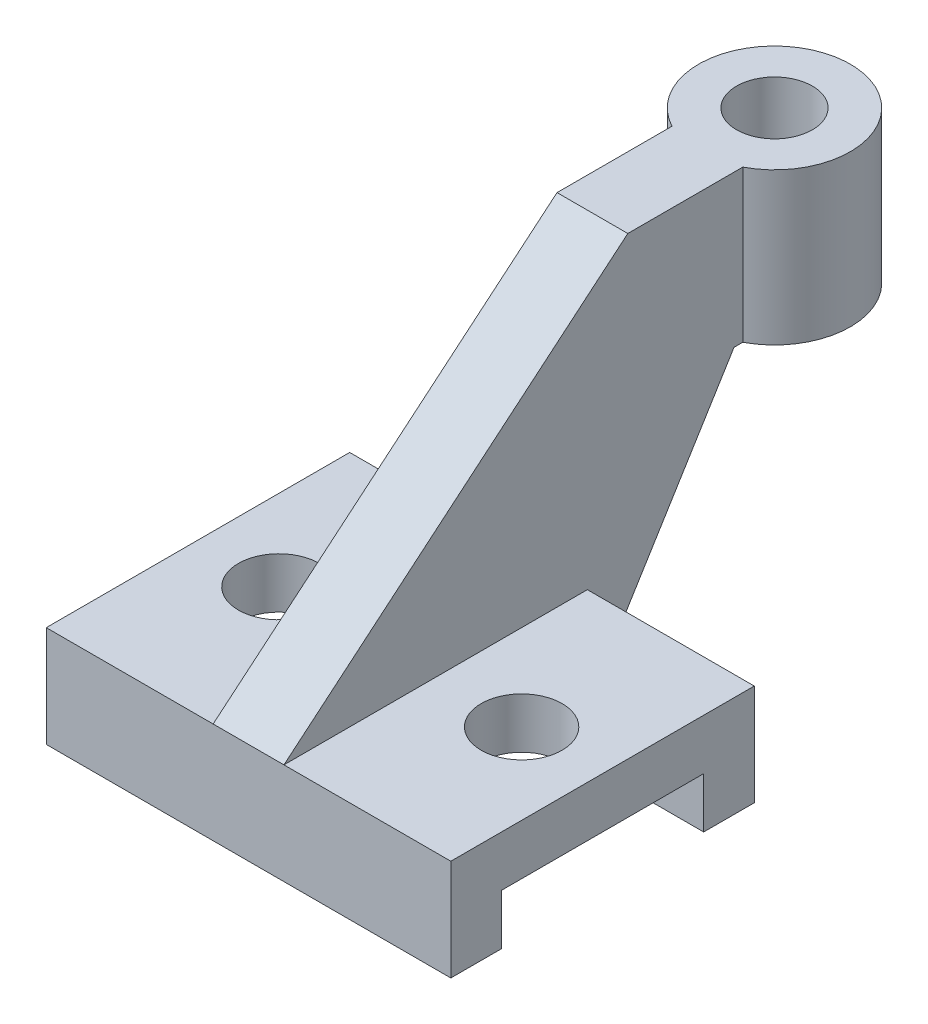
ISO-10303-21;
HEADER;
FILE_DESCRIPTION(('STEP AP214'),'2;1');
FILE_NAME('part.step','',(''),(''),'','','');
FILE_SCHEMA(('AUTOMOTIVE_DESIGN { 1 0 10303 214 1 1 1 1 }'));
ENDSEC;
DATA;
#1=APPLICATION_CONTEXT('core data for automotive mechanical design processes');
#2=APPLICATION_PROTOCOL_DEFINITION('international standard','automotive_design',2000,#1);
#3=PRODUCT_CONTEXT('',#1,'mechanical');
#4=PRODUCT('Part','Part','',(#3));
#5=PRODUCT_RELATED_PRODUCT_CATEGORY('part','',(#4));
#6=PRODUCT_DEFINITION_FORMATION('','',#4);
#7=PRODUCT_DEFINITION_CONTEXT('part definition',#1,'design');
#8=PRODUCT_DEFINITION('design','',#6,#7);
#9=PRODUCT_DEFINITION_SHAPE('','',#8);
#10=(LENGTH_UNIT() NAMED_UNIT(*) SI_UNIT(.MILLI.,.METRE.));
#11=(NAMED_UNIT(*) PLANE_ANGLE_UNIT() SI_UNIT($,.RADIAN.));
#12=(NAMED_UNIT(*) SI_UNIT($,.STERADIAN.) SOLID_ANGLE_UNIT());
#13=UNCERTAINTY_MEASURE_WITH_UNIT(LENGTH_MEASURE(1.E-05),#10,'distance_accuracy_value','');
#14=(GEOMETRIC_REPRESENTATION_CONTEXT(3) GLOBAL_UNCERTAINTY_ASSIGNED_CONTEXT((#13)) GLOBAL_UNIT_ASSIGNED_CONTEXT((#10,
#11,#12)) REPRESENTATION_CONTEXT('',''));
#15=CARTESIAN_POINT('',(0.,0.,0.));
#16=DIRECTION('',(0.,0.,1.));
#17=DIRECTION('',(1.,0.,0.));
#18=AXIS2_PLACEMENT_3D('',#15,#16,#17);
#19=CARTESIAN_POINT('',(-40.,-10.,30.));
#20=DIRECTION('',(0.,1.,0.));
#21=DIRECTION('',(0.,0.,1.));
#22=AXIS2_PLACEMENT_3D('',#19,#20,#21);
#23=PLANE('',#22);
#24=DIRECTION('',(1.,0.,0.));
#25=VECTOR('',#24,1.);
#26=CARTESIAN_POINT('',(-40.,-10.,-20.));
#27=LINE('',#26,#25);
#28=CARTESIAN_POINT('',(-40.,-10.,-20.));
#29=VERTEX_POINT('',#28);
#30=CARTESIAN_POINT('',(40.,-10.,-20.));
#31=VERTEX_POINT('',#30);
#32=EDGE_CURVE('E154',#29,#31,#27,.T.);
#33=ORIENTED_EDGE('',*,*,#32,.F.);
#34=DIRECTION('',(0.,0.,-1.));
#35=VECTOR('',#34,1.);
#36=CARTESIAN_POINT('',(-40.,-10.,30.));
#37=LINE('',#36,#35);
#38=CARTESIAN_POINT('',(-40.,-10.,-30.));
#39=VERTEX_POINT('',#38);
#40=EDGE_CURVE('E172',#29,#39,#37,.T.);
#41=ORIENTED_EDGE('',*,*,#40,.T.);
#42=DIRECTION('',(1.,0.,0.));
#43=VECTOR('',#42,1.);
#44=CARTESIAN_POINT('',(-40.,-10.,-30.));
#45=LINE('',#44,#43);
#46=CARTESIAN_POINT('',(-7.,-10.,-30.));
#47=VERTEX_POINT('',#46);
#48=EDGE_CURVE('E269',#39,#47,#45,.T.);
#49=ORIENTED_EDGE('',*,*,#48,.T.);
#50=DIRECTION('',(-1.,0.,0.));
#51=VECTOR('',#50,1.);
#52=CARTESIAN_POINT('',(7.,-10.,-30.));
#53=LINE('',#52,#51);
#54=CARTESIAN_POINT('',(7.,-10.,-30.));
#55=VERTEX_POINT('',#54);
#56=EDGE_CURVE('E265',#55,#47,#53,.T.);
#57=ORIENTED_EDGE('',*,*,#56,.F.);
#58=CARTESIAN_POINT('',(40.,-10.,-30.));
#59=VERTEX_POINT('',#58);
#60=EDGE_CURVE('E286',#55,#59,#45,.T.);
#61=ORIENTED_EDGE('',*,*,#60,.T.);
#62=DIRECTION('',(0.,0.,-1.));
#63=VECTOR('',#62,1.);
#64=CARTESIAN_POINT('',(40.,-10.,30.));
#65=LINE('',#64,#63);
#66=EDGE_CURVE('E280',#31,#59,#65,.T.);
#67=ORIENTED_EDGE('',*,*,#66,.F.);
#68=EDGE_LOOP('',(#33,#41,#49,#57,#61,#67));
#69=FACE_BOUND('',#68,.T.);
#70=ADVANCED_FACE('F39',(#69),#23,.F.);
#71=CARTESIAN_POINT('',(40.,10.,30.));
#72=DIRECTION('',(-1.,0.,0.));
#73=DIRECTION('',(0.,0.,1.));
#74=AXIS2_PLACEMENT_3D('',#71,#72,#73);
#75=PLANE('',#74);
#76=DIRECTION('',(0.,-1.,0.));
#77=VECTOR('',#76,1.);
#78=CARTESIAN_POINT('',(40.,-10.,20.));
#79=LINE('',#78,#77);
#80=CARTESIAN_POINT('',(40.,0.,20.));
#81=VERTEX_POINT('',#80);
#82=CARTESIAN_POINT('',(40.,-10.,20.));
#83=VERTEX_POINT('',#82);
#84=EDGE_CURVE('E147',#81,#83,#79,.T.);
#85=ORIENTED_EDGE('',*,*,#84,.F.);
#86=DIRECTION('',(0.,0.,1.));
#87=VECTOR('',#86,1.);
#88=CARTESIAN_POINT('',(40.,0.,20.));
#89=LINE('',#88,#87);
#90=CARTESIAN_POINT('',(40.,0.,-20.));
#91=VERTEX_POINT('',#90);
#92=EDGE_CURVE('E169',#91,#81,#89,.T.);
#93=ORIENTED_EDGE('',*,*,#92,.F.);
#94=DIRECTION('',(0.,1.,0.));
#95=VECTOR('',#94,1.);
#96=CARTESIAN_POINT('',(40.,-10.,-20.));
#97=LINE('',#96,#95);
#98=EDGE_CURVE('E225',#31,#91,#97,.T.);
#99=ORIENTED_EDGE('',*,*,#98,.F.);
#100=ORIENTED_EDGE('',*,*,#66,.T.);
#101=DIRECTION('',(0.,1.,0.));
#102=VECTOR('',#101,1.);
#103=CARTESIAN_POINT('',(40.,10.,-30.));
#104=LINE('',#103,#102);
#105=CARTESIAN_POINT('',(40.,10.,-30.));
#106=VERTEX_POINT('',#105);
#107=EDGE_CURVE('E264',#59,#106,#104,.T.);
#108=ORIENTED_EDGE('',*,*,#107,.T.);
#109=DIRECTION('',(0.,0.,-1.));
#110=VECTOR('',#109,1.);
#111=CARTESIAN_POINT('',(40.,10.,30.));
#112=LINE('',#111,#110);
#113=CARTESIAN_POINT('',(40.,10.,30.));
#114=VERTEX_POINT('',#113);
#115=EDGE_CURVE('E176',#114,#106,#112,.T.);
#116=ORIENTED_EDGE('',*,*,#115,.F.);
#117=DIRECTION('',(0.,1.,0.));
#118=VECTOR('',#117,1.);
#119=CARTESIAN_POINT('',(40.,10.,30.));
#120=LINE('',#119,#118);
#121=CARTESIAN_POINT('',(40.,-10.,30.));
#122=VERTEX_POINT('',#121);
#123=EDGE_CURVE('E266',#122,#114,#120,.T.);
#124=ORIENTED_EDGE('',*,*,#123,.F.);
#125=EDGE_CURVE('E178',#122,#83,#65,.T.);
#126=ORIENTED_EDGE('',*,*,#125,.T.);
#127=EDGE_LOOP('',(#85,#93,#99,#100,#108,#116,#124,#126));
#128=FACE_BOUND('',#127,.T.);
#129=ADVANCED_FACE('F300',(#128),#75,.F.);
#130=CARTESIAN_POINT('',(0.,37.,-74.));
#131=DIRECTION('',(0.,1.,0.));
#132=DIRECTION('',(0.,0.,1.));
#133=AXIS2_PLACEMENT_3D('',#130,#131,#132);
#134=PLANE('',#133);
#135=CARTESIAN_POINT('',(0.,37.,-74.));
#136=DIRECTION('',(0.,1.,0.));
#137=DIRECTION('',(0.,0.,1.));
#138=AXIS2_PLACEMENT_3D('',#135,#136,#137);
#139=CIRCLE('',#138,7.5);
#140=CARTESIAN_POINT('',(0.,37.,-66.5));
#141=VERTEX_POINT('',#140);
#142=EDGE_CURVE('E200',#141,#141,#139,.T.);
#143=ORIENTED_EDGE('',*,*,#142,.T.);
#144=EDGE_LOOP('',(#143));
#145=FACE_BOUND('',#144,.T.);
#146=DIRECTION('',(-1.,0.,0.));
#147=VECTOR('',#146,1.);
#148=CARTESIAN_POINT('',(7.,37.,-59.));
#149=LINE('',#148,#147);
#150=CARTESIAN_POINT('',(7.,37.,-59.));
#151=VERTEX_POINT('',#150);
#152=CARTESIAN_POINT('',(-7.,37.,-59.));
#153=VERTEX_POINT('',#152);
#154=EDGE_CURVE('E65',#151,#153,#149,.T.);
#155=ORIENTED_EDGE('',*,*,#154,.T.);
#156=DIRECTION('',(0.,0.,1.));
#157=VECTOR('',#156,1.);
#158=CARTESIAN_POINT('',(-7.,37.,-66.));
#159=LINE('',#158,#157);
#160=CARTESIAN_POINT('',(-7.,37.,-60.7335008385784));
#161=VERTEX_POINT('',#160);
#162=EDGE_CURVE('E187',#161,#153,#159,.T.);
#163=ORIENTED_EDGE('',*,*,#162,.F.);
#164=CARTESIAN_POINT('',(0.,37.,-74.));
#165=DIRECTION('',(0.,1.,0.));
#166=DIRECTION('',(0.,0.,1.));
#167=AXIS2_PLACEMENT_3D('',#164,#165,#166);
#168=CIRCLE('',#167,15.);
#169=CARTESIAN_POINT('',(7.,37.,-60.7335008385784));
#170=VERTEX_POINT('',#169);
#171=EDGE_CURVE('E11',#170,#161,#168,.T.);
#172=ORIENTED_EDGE('',*,*,#171,.F.);
#173=DIRECTION('',(0.,0.,1.));
#174=VECTOR('',#173,1.);
#175=CARTESIAN_POINT('',(7.,37.,-66.));
#176=LINE('',#175,#174);
#177=EDGE_CURVE('E186',#170,#151,#176,.T.);
#178=ORIENTED_EDGE('',*,*,#177,.T.);
#179=EDGE_LOOP('',(#155,#163,#172,#178));
#180=FACE_BOUND('',#179,.T.);
#181=ADVANCED_FACE('F344',(#145,#180),#134,.F.);
#182=CARTESIAN_POINT('',(0.,37.,-74.));
#183=DIRECTION('',(0.,1.,0.));
#184=DIRECTION('',(0.,0.,1.));
#185=AXIS2_PLACEMENT_3D('',#182,#183,#184);
#186=CYLINDRICAL_SURFACE('',#185,15.);
#187=CARTESIAN_POINT('',(0.,67.,-74.));
#188=DIRECTION('',(0.,1.,0.));
#189=DIRECTION('',(0.,0.,1.));
#190=AXIS2_PLACEMENT_3D('',#187,#188,#189);
#191=CIRCLE('',#190,15.);
#192=CARTESIAN_POINT('',(7.,67.,-60.7335008385784));
#193=VERTEX_POINT('',#192);
#194=CARTESIAN_POINT('',(-7.,67.,-60.7335008385784));
#195=VERTEX_POINT('',#194);
#196=EDGE_CURVE('E48',#193,#195,#191,.T.);
#197=ORIENTED_EDGE('',*,*,#196,.F.);
#198=DIRECTION('',(0.,1.,0.));
#199=VECTOR('',#198,1.);
#200=CARTESIAN_POINT('',(7.,37.,-60.7335008385784));
#201=LINE('',#200,#199);
#202=EDGE_CURVE('E194',#193,#170,#201,.F.);
#203=ORIENTED_EDGE('',*,*,#202,.T.);
#204=ORIENTED_EDGE('',*,*,#171,.T.);
#205=DIRECTION('',(0.,1.,0.));
#206=VECTOR('',#205,1.);
#207=CARTESIAN_POINT('',(-7.,37.,-60.7335008385784));
#208=LINE('',#207,#206);
#209=EDGE_CURVE('E195',#161,#195,#208,.T.);
#210=ORIENTED_EDGE('',*,*,#209,.T.);
#211=EDGE_LOOP('',(#197,#203,#204,#210));
#212=FACE_BOUND('',#211,.T.);
#213=ADVANCED_FACE('F41',(#212),#186,.T.);
#214=CARTESIAN_POINT('',(0.,67.,-74.));
#215=DIRECTION('',(0.,1.,0.));
#216=DIRECTION('',(0.,0.,1.));
#217=AXIS2_PLACEMENT_3D('',#214,#215,#216);
#218=PLANE('',#217);
#219=DIRECTION('',(0.,0.,1.));
#220=VECTOR('',#219,1.);
#221=CARTESIAN_POINT('',(-7.,67.,-66.));
#222=LINE('',#221,#220);
#223=CARTESIAN_POINT('',(-7.,67.,-38.));
#224=VERTEX_POINT('',#223);
#225=EDGE_CURVE('E188',#195,#224,#222,.T.);
#226=ORIENTED_EDGE('',*,*,#225,.T.);
#227=DIRECTION('',(-1.,0.,0.));
#228=VECTOR('',#227,1.);
#229=CARTESIAN_POINT('',(7.,67.,-38.));
#230=LINE('',#229,#228);
#231=CARTESIAN_POINT('',(7.,67.,-38.));
#232=VERTEX_POINT('',#231);
#233=EDGE_CURVE('E256',#232,#224,#230,.T.);
#234=ORIENTED_EDGE('',*,*,#233,.F.);
#235=DIRECTION('',(0.,0.,1.));
#236=VECTOR('',#235,1.);
#237=CARTESIAN_POINT('',(7.,67.,-66.));
#238=LINE('',#237,#236);
#239=EDGE_CURVE('E184',#193,#232,#238,.T.);
#240=ORIENTED_EDGE('',*,*,#239,.F.);
#241=ORIENTED_EDGE('',*,*,#196,.T.);
#242=EDGE_LOOP('',(#226,#234,#240,#241));
#243=FACE_BOUND('',#242,.T.);
#244=CARTESIAN_POINT('',(0.,67.,-74.));
#245=DIRECTION('',(0.,1.,0.));
#246=DIRECTION('',(0.,0.,1.));
#247=AXIS2_PLACEMENT_3D('',#244,#245,#246);
#248=CIRCLE('',#247,7.5);
#249=CARTESIAN_POINT('',(0.,67.,-66.5));
#250=VERTEX_POINT('',#249);
#251=EDGE_CURVE('E196',#250,#250,#248,.T.);
#252=ORIENTED_EDGE('',*,*,#251,.F.);
#253=EDGE_LOOP('',(#252));
#254=FACE_BOUND('',#253,.T.);
#255=ADVANCED_FACE('F478',(#243,#254),#218,.T.);
#256=CARTESIAN_POINT('',(0.,37.,-74.));
#257=DIRECTION('',(0.,1.,0.));
#258=DIRECTION('',(0.,0.,1.));
#259=AXIS2_PLACEMENT_3D('',#256,#257,#258);
#260=CYLINDRICAL_SURFACE('',#259,7.5);
#261=ORIENTED_EDGE('',*,*,#142,.F.);
#262=EDGE_LOOP('',(#261));
#263=FACE_BOUND('',#262,.T.);
#264=ORIENTED_EDGE('',*,*,#251,.T.);
#265=EDGE_LOOP('',(#264));
#266=FACE_BOUND('',#265,.T.);
#267=ADVANCED_FACE('F472',(#263,#266),#260,.F.);
#268=CARTESIAN_POINT('',(7.,67.,-66.));
#269=DIRECTION('',(-1.,0.,0.));
#270=DIRECTION('',(0.,0.,1.));
#271=AXIS2_PLACEMENT_3D('',#268,#269,#270);
#272=PLANE('',#271);
#273=ORIENTED_EDGE('',*,*,#239,.T.);
#274=DIRECTION('',(0.,-0.642398813226134,0.76637051402416));
#275=VECTOR('',#274,1.);
#276=CARTESIAN_POINT('',(7.,10.,30.));
#277=LINE('',#276,#275);
#278=CARTESIAN_POINT('',(7.,10.,30.));
#279=VERTEX_POINT('',#278);
#280=EDGE_CURVE('E242',#232,#279,#277,.T.);
#281=ORIENTED_EDGE('',*,*,#280,.T.);
#282=DIRECTION('',(0.,0.,-1.));
#283=VECTOR('',#282,1.);
#284=CARTESIAN_POINT('',(7.,10.,30.));
#285=LINE('',#284,#283);
#286=CARTESIAN_POINT('',(7.,10.,-30.));
#287=VERTEX_POINT('',#286);
#288=EDGE_CURVE('E233',#279,#287,#285,.T.);
#289=ORIENTED_EDGE('',*,*,#288,.T.);
#290=DIRECTION('',(0.,-1.,0.));
#291=VECTOR('',#290,1.);
#292=CARTESIAN_POINT('',(7.,-10.,-30.));
#293=LINE('',#292,#291);
#294=EDGE_CURVE('E237',#287,#55,#293,.T.);
#295=ORIENTED_EDGE('',*,*,#294,.T.);
#296=DIRECTION('',(0.,0.851036012799674,-0.525107327046607));
#297=VECTOR('',#296,1.);
#298=CARTESIAN_POINT('',(7.,-10.,-30.));
#299=LINE('',#298,#297);
#300=EDGE_CURVE('E238',#55,#151,#299,.T.);
#301=ORIENTED_EDGE('',*,*,#300,.T.);
#302=ORIENTED_EDGE('',*,*,#177,.F.);
#303=ORIENTED_EDGE('',*,*,#202,.F.);
#304=EDGE_LOOP('',(#273,#281,#289,#295,#301,#302,#303));
#305=FACE_BOUND('',#304,.T.);
#306=ADVANCED_FACE('F321',(#305),#272,.F.);
#307=CARTESIAN_POINT('',(-7.,37.,-66.));
#308=DIRECTION('',(1.,0.,0.));
#309=DIRECTION('',(0.,0.,-1.));
#310=AXIS2_PLACEMENT_3D('',#307,#308,#309);
#311=PLANE('',#310);
#312=ORIENTED_EDGE('',*,*,#162,.T.);
#313=DIRECTION('',(0.,0.851036012799674,-0.525107327046607));
#314=VECTOR('',#313,1.);
#315=CARTESIAN_POINT('',(-7.,-10.,-30.));
#316=LINE('',#315,#314);
#317=EDGE_CURVE('E253',#47,#153,#316,.T.);
#318=ORIENTED_EDGE('',*,*,#317,.F.);
#319=DIRECTION('',(0.,-1.,0.));
#320=VECTOR('',#319,1.);
#321=CARTESIAN_POINT('',(-7.,-10.,-30.));
#322=LINE('',#321,#320);
#323=CARTESIAN_POINT('',(-7.,10.,-30.));
#324=VERTEX_POINT('',#323);
#325=EDGE_CURVE('E247',#324,#47,#322,.T.);
#326=ORIENTED_EDGE('',*,*,#325,.F.);
#327=DIRECTION('',(0.,0.,-1.));
#328=VECTOR('',#327,1.);
#329=CARTESIAN_POINT('',(-7.,10.,30.));
#330=LINE('',#329,#328);
#331=CARTESIAN_POINT('',(-7.,10.,30.));
#332=VERTEX_POINT('',#331);
#333=EDGE_CURVE('E230',#332,#324,#330,.T.);
#334=ORIENTED_EDGE('',*,*,#333,.F.);
#335=DIRECTION('',(0.,-0.642398813226134,0.76637051402416));
#336=VECTOR('',#335,1.);
#337=CARTESIAN_POINT('',(-7.,10.,30.));
#338=LINE('',#337,#336);
#339=EDGE_CURVE('E240',#224,#332,#338,.T.);
#340=ORIENTED_EDGE('',*,*,#339,.F.);
#341=ORIENTED_EDGE('',*,*,#225,.F.);
#342=ORIENTED_EDGE('',*,*,#209,.F.);
#343=EDGE_LOOP('',(#312,#318,#326,#334,#340,#341,#342));
#344=FACE_BOUND('',#343,.T.);
#345=ADVANCED_FACE('F312',(#344),#311,.F.);
#346=CARTESIAN_POINT('',(-40.,10.,30.));
#347=DIRECTION('',(0.,-1.,0.));
#348=DIRECTION('',(0.,0.,-1.));
#349=AXIS2_PLACEMENT_3D('',#346,#347,#348);
#350=PLANE('',#349);
#351=CARTESIAN_POINT('',(-24.,10.,0.));
#352=DIRECTION('',(0.,1.,0.));
#353=DIRECTION('',(0.,0.,1.));
#354=AXIS2_PLACEMENT_3D('',#351,#352,#353);
#355=CIRCLE('',#354,8.);
#356=CARTESIAN_POINT('',(-24.,10.,8.));
#357=VERTEX_POINT('',#356);
#358=EDGE_CURVE('E210',#357,#357,#355,.T.);
#359=ORIENTED_EDGE('',*,*,#358,.F.);
#360=EDGE_LOOP('',(#359));
#361=FACE_BOUND('',#360,.T.);
#362=ORIENTED_EDGE('',*,*,#333,.T.);
#363=DIRECTION('',(-1.,0.,0.));
#364=VECTOR('',#363,1.);
#365=CARTESIAN_POINT('',(-40.,10.,-30.));
#366=LINE('',#365,#364);
#367=CARTESIAN_POINT('',(-40.,10.,-30.));
#368=VERTEX_POINT('',#367);
#369=EDGE_CURVE('E278',#324,#368,#366,.T.);
#370=ORIENTED_EDGE('',*,*,#369,.T.);
#371=DIRECTION('',(0.,0.,-1.));
#372=VECTOR('',#371,1.);
#373=CARTESIAN_POINT('',(-40.,10.,30.));
#374=LINE('',#373,#372);
#375=CARTESIAN_POINT('',(-40.,10.,30.));
#376=VERTEX_POINT('',#375);
#377=EDGE_CURVE('E174',#376,#368,#374,.T.);
#378=ORIENTED_EDGE('',*,*,#377,.F.);
#379=DIRECTION('',(-1.,0.,0.));
#380=VECTOR('',#379,1.);
#381=CARTESIAN_POINT('',(-40.,10.,30.));
#382=LINE('',#381,#380);
#383=EDGE_CURVE('E267',#332,#376,#382,.T.);
#384=ORIENTED_EDGE('',*,*,#383,.F.);
#385=EDGE_LOOP('',(#362,#370,#378,#384));
#386=FACE_BOUND('',#385,.T.);
#387=ADVANCED_FACE('F330',(#361,#386),#350,.F.);
#388=CARTESIAN_POINT('',(0.,0.,-30.));
#389=DIRECTION('',(0.,0.,1.));
#390=DIRECTION('',(1.,0.,0.));
#391=AXIS2_PLACEMENT_3D('',#388,#389,#390);
#392=PLANE('',#391);
#393=ORIENTED_EDGE('',*,*,#325,.T.);
#394=ORIENTED_EDGE('',*,*,#48,.F.);
#395=DIRECTION('',(0.,-1.,0.));
#396=VECTOR('',#395,1.);
#397=CARTESIAN_POINT('',(-40.,10.,-30.));
#398=LINE('',#397,#396);
#399=EDGE_CURVE('E285',#368,#39,#398,.T.);
#400=ORIENTED_EDGE('',*,*,#399,.F.);
#401=ORIENTED_EDGE('',*,*,#369,.F.);
#402=EDGE_LOOP('',(#393,#394,#400,#401));
#403=FACE_BOUND('',#402,.T.);
#404=ADVANCED_FACE('F309',(#403),#392,.F.);
#405=CARTESIAN_POINT('',(24.,10.,0.));
#406=DIRECTION('',(0.,1.,0.));
#407=DIRECTION('',(0.,0.,1.));
#408=AXIS2_PLACEMENT_3D('',#405,#406,#407);
#409=CIRCLE('',#408,8.);
#410=CARTESIAN_POINT('',(24.,10.,8.));
#411=VERTEX_POINT('',#410);
#412=EDGE_CURVE('E215',#411,#411,#409,.T.);
#413=ORIENTED_EDGE('',*,*,#412,.F.);
#414=EDGE_LOOP('',(#413));
#415=FACE_BOUND('',#414,.T.);
#416=EDGE_CURVE('E283',#106,#287,#366,.T.);
#417=ORIENTED_EDGE('',*,*,#416,.T.);
#418=ORIENTED_EDGE('',*,*,#288,.F.);
#419=EDGE_CURVE('E271',#114,#279,#382,.T.);
#420=ORIENTED_EDGE('',*,*,#419,.F.);
#421=ORIENTED_EDGE('',*,*,#115,.T.);
#422=EDGE_LOOP('',(#417,#418,#420,#421));
#423=FACE_BOUND('',#422,.T.);
#424=ADVANCED_FACE('F323',(#415,#423),#350,.F.);
#425=CARTESIAN_POINT('',(-40.,10.,30.));
#426=DIRECTION('',(1.,0.,0.));
#427=DIRECTION('',(0.,0.,-1.));
#428=AXIS2_PLACEMENT_3D('',#425,#426,#427);
#429=PLANE('',#428);
#430=DIRECTION('',(0.,0.,1.));
#431=VECTOR('',#430,1.);
#432=CARTESIAN_POINT('',(-40.,0.,20.));
#433=LINE('',#432,#431);
#434=CARTESIAN_POINT('',(-40.,0.,-20.));
#435=VERTEX_POINT('',#434);
#436=CARTESIAN_POINT('',(-40.,0.,20.));
#437=VERTEX_POINT('',#436);
#438=EDGE_CURVE('E156',#435,#437,#433,.T.);
#439=ORIENTED_EDGE('',*,*,#438,.T.);
#440=DIRECTION('',(0.,-1.,0.));
#441=VECTOR('',#440,1.);
#442=CARTESIAN_POINT('',(-40.,-10.,20.));
#443=LINE('',#442,#441);
#444=CARTESIAN_POINT('',(-40.,-10.,20.));
#445=VERTEX_POINT('',#444);
#446=EDGE_CURVE('E57',#437,#445,#443,.T.);
#447=ORIENTED_EDGE('',*,*,#446,.T.);
#448=CARTESIAN_POINT('',(-40.,-10.,30.));
#449=VERTEX_POINT('',#448);
#450=EDGE_CURVE('E162',#449,#445,#37,.T.);
#451=ORIENTED_EDGE('',*,*,#450,.F.);
#452=DIRECTION('',(0.,-1.,0.));
#453=VECTOR('',#452,1.);
#454=CARTESIAN_POINT('',(-40.,10.,30.));
#455=LINE('',#454,#453);
#456=EDGE_CURVE('E273',#376,#449,#455,.T.);
#457=ORIENTED_EDGE('',*,*,#456,.F.);
#458=ORIENTED_EDGE('',*,*,#377,.T.);
#459=ORIENTED_EDGE('',*,*,#399,.T.);
#460=ORIENTED_EDGE('',*,*,#40,.F.);
#461=DIRECTION('',(0.,1.,0.));
#462=VECTOR('',#461,1.);
#463=CARTESIAN_POINT('',(-40.,-10.,-20.));
#464=LINE('',#463,#462);
#465=EDGE_CURVE('E170',#29,#435,#464,.T.);
#466=ORIENTED_EDGE('',*,*,#465,.T.);
#467=EDGE_LOOP('',(#439,#447,#451,#457,#458,#459,#460,#466));
#468=FACE_BOUND('',#467,.T.);
#469=ADVANCED_FACE('F161',(#468),#429,.F.);
#470=ORIENTED_EDGE('',*,*,#450,.T.);
#471=DIRECTION('',(1.,0.,0.));
#472=VECTOR('',#471,1.);
#473=CARTESIAN_POINT('',(-40.,-10.,20.));
#474=LINE('',#473,#472);
#475=EDGE_CURVE('E150',#445,#83,#474,.T.);
#476=ORIENTED_EDGE('',*,*,#475,.T.);
#477=ORIENTED_EDGE('',*,*,#125,.F.);
#478=DIRECTION('',(1.,0.,0.));
#479=VECTOR('',#478,1.);
#480=CARTESIAN_POINT('',(-40.,-10.,30.));
#481=LINE('',#480,#479);
#482=EDGE_CURVE('E173',#449,#122,#481,.T.);
#483=ORIENTED_EDGE('',*,*,#482,.F.);
#484=EDGE_LOOP('',(#470,#476,#477,#483));
#485=FACE_BOUND('',#484,.T.);
#486=ADVANCED_FACE('F168',(#485),#23,.F.);
#487=CARTESIAN_POINT('',(0.,0.,30.));
#488=DIRECTION('',(0.,0.,1.));
#489=DIRECTION('',(1.,0.,0.));
#490=AXIS2_PLACEMENT_3D('',#487,#488,#489);
#491=PLANE('',#490);
#492=ORIENTED_EDGE('',*,*,#123,.T.);
#493=ORIENTED_EDGE('',*,*,#419,.T.);
#494=DIRECTION('',(-1.,0.,0.));
#495=VECTOR('',#494,1.);
#496=CARTESIAN_POINT('',(7.,10.,30.));
#497=LINE('',#496,#495);
#498=EDGE_CURVE('E246',#279,#332,#497,.T.);
#499=ORIENTED_EDGE('',*,*,#498,.T.);
#500=ORIENTED_EDGE('',*,*,#383,.T.);
#501=ORIENTED_EDGE('',*,*,#456,.T.);
#502=ORIENTED_EDGE('',*,*,#482,.T.);
#503=EDGE_LOOP('',(#492,#493,#499,#500,#501,#502));
#504=FACE_BOUND('',#503,.T.);
#505=ADVANCED_FACE('F302',(#504),#491,.T.);
#506=ORIENTED_EDGE('',*,*,#60,.F.);
#507=ORIENTED_EDGE('',*,*,#294,.F.);
#508=ORIENTED_EDGE('',*,*,#416,.F.);
#509=ORIENTED_EDGE('',*,*,#107,.F.);
#510=EDGE_LOOP('',(#506,#507,#508,#509));
#511=FACE_BOUND('',#510,.T.);
#512=ADVANCED_FACE('F298',(#511),#392,.F.);
#513=CARTESIAN_POINT('',(7.,-10.,-30.));
#514=DIRECTION('',(0.,0.525107327046607,0.851036012799674));
#515=DIRECTION('',(0.,-0.851036012799674,0.525107327046607));
#516=AXIS2_PLACEMENT_3D('',#513,#514,#515);
#517=PLANE('',#516);
#518=ORIENTED_EDGE('',*,*,#317,.T.);
#519=ORIENTED_EDGE('',*,*,#154,.F.);
#520=ORIENTED_EDGE('',*,*,#300,.F.);
#521=ORIENTED_EDGE('',*,*,#56,.T.);
#522=EDGE_LOOP('',(#518,#519,#520,#521));
#523=FACE_BOUND('',#522,.T.);
#524=ADVANCED_FACE('F318',(#523),#517,.F.);
#525=CARTESIAN_POINT('',(7.,10.,30.));
#526=DIRECTION('',(0.,-0.76637051402416,-0.642398813226134));
#527=DIRECTION('',(0.,0.642398813226134,-0.76637051402416));
#528=AXIS2_PLACEMENT_3D('',#525,#526,#527);
#529=PLANE('',#528);
#530=ORIENTED_EDGE('',*,*,#339,.T.);
#531=ORIENTED_EDGE('',*,*,#498,.F.);
#532=ORIENTED_EDGE('',*,*,#280,.F.);
#533=ORIENTED_EDGE('',*,*,#233,.T.);
#534=EDGE_LOOP('',(#530,#531,#532,#533));
#535=FACE_BOUND('',#534,.T.);
#536=ADVANCED_FACE('F358',(#535),#529,.F.);
#537=CARTESIAN_POINT('',(-40.,-10.,20.));
#538=DIRECTION('',(0.,0.,1.));
#539=DIRECTION('',(1.,0.,0.));
#540=AXIS2_PLACEMENT_3D('',#537,#538,#539);
#541=PLANE('',#540);
#542=ORIENTED_EDGE('',*,*,#84,.T.);
#543=ORIENTED_EDGE('',*,*,#475,.F.);
#544=ORIENTED_EDGE('',*,*,#446,.F.);
#545=DIRECTION('',(1.,0.,0.));
#546=VECTOR('',#545,1.);
#547=CARTESIAN_POINT('',(-40.,0.,20.));
#548=LINE('',#547,#546);
#549=EDGE_CURVE('E229',#437,#81,#548,.T.);
#550=ORIENTED_EDGE('',*,*,#549,.T.);
#551=EDGE_LOOP('',(#542,#543,#544,#550));
#552=FACE_BOUND('',#551,.T.);
#553=ADVANCED_FACE('F146',(#552),#541,.F.);
#554=CARTESIAN_POINT('',(-40.,0.,20.));
#555=DIRECTION('',(0.,1.,0.));
#556=DIRECTION('',(0.,0.,1.));
#557=AXIS2_PLACEMENT_3D('',#554,#555,#556);
#558=PLANE('',#557);
#559=CARTESIAN_POINT('',(-24.,0.,0.));
#560=DIRECTION('',(0.,1.,0.));
#561=DIRECTION('',(0.,0.,1.));
#562=AXIS2_PLACEMENT_3D('',#559,#560,#561);
#563=CIRCLE('',#562,8.);
#564=CARTESIAN_POINT('',(-24.,0.,8.));
#565=VERTEX_POINT('',#564);
#566=EDGE_CURVE('E43',#565,#565,#563,.T.);
#567=ORIENTED_EDGE('',*,*,#566,.T.);
#568=EDGE_LOOP('',(#567));
#569=FACE_BOUND('',#568,.T.);
#570=CARTESIAN_POINT('',(24.,0.,0.));
#571=DIRECTION('',(0.,1.,0.));
#572=DIRECTION('',(0.,0.,1.));
#573=AXIS2_PLACEMENT_3D('',#570,#571,#572);
#574=CIRCLE('',#573,8.);
#575=CARTESIAN_POINT('',(24.,0.,8.));
#576=VERTEX_POINT('',#575);
#577=EDGE_CURVE('E202',#576,#576,#574,.T.);
#578=ORIENTED_EDGE('',*,*,#577,.T.);
#579=EDGE_LOOP('',(#578));
#580=FACE_BOUND('',#579,.T.);
#581=ORIENTED_EDGE('',*,*,#92,.T.);
#582=ORIENTED_EDGE('',*,*,#549,.F.);
#583=ORIENTED_EDGE('',*,*,#438,.F.);
#584=DIRECTION('',(1.,0.,0.));
#585=VECTOR('',#584,1.);
#586=CARTESIAN_POINT('',(-40.,0.,-20.));
#587=LINE('',#586,#585);
#588=EDGE_CURVE('E226',#435,#91,#587,.T.);
#589=ORIENTED_EDGE('',*,*,#588,.T.);
#590=EDGE_LOOP('',(#581,#582,#583,#589));
#591=FACE_BOUND('',#590,.T.);
#592=ADVANCED_FACE('F362',(#569,#580,#591),#558,.F.);
#593=CARTESIAN_POINT('',(-40.,-10.,-20.));
#594=DIRECTION('',(0.,0.,-1.));
#595=DIRECTION('',(-1.,0.,0.));
#596=AXIS2_PLACEMENT_3D('',#593,#594,#595);
#597=PLANE('',#596);
#598=ORIENTED_EDGE('',*,*,#98,.T.);
#599=ORIENTED_EDGE('',*,*,#588,.F.);
#600=ORIENTED_EDGE('',*,*,#465,.F.);
#601=ORIENTED_EDGE('',*,*,#32,.T.);
#602=EDGE_LOOP('',(#598,#599,#600,#601));
#603=FACE_BOUND('',#602,.T.);
#604=ADVANCED_FACE('F361',(#603),#597,.F.);
#605=CARTESIAN_POINT('',(24.,-10.,0.));
#606=DIRECTION('',(0.,1.,0.));
#607=DIRECTION('',(0.,0.,1.));
#608=AXIS2_PLACEMENT_3D('',#605,#606,#607);
#609=CYLINDRICAL_SURFACE('',#608,8.);
#610=ORIENTED_EDGE('',*,*,#412,.T.);
#611=EDGE_LOOP('',(#610));
#612=FACE_BOUND('',#611,.T.);
#613=ORIENTED_EDGE('',*,*,#577,.F.);
#614=EDGE_LOOP('',(#613));
#615=FACE_BOUND('',#614,.T.);
#616=ADVANCED_FACE('F368',(#612,#615),#609,.F.);
#617=CARTESIAN_POINT('',(-24.,-10.,0.));
#618=DIRECTION('',(0.,1.,0.));
#619=DIRECTION('',(0.,0.,1.));
#620=AXIS2_PLACEMENT_3D('',#617,#618,#619);
#621=CYLINDRICAL_SURFACE('',#620,8.);
#622=ORIENTED_EDGE('',*,*,#358,.T.);
#623=EDGE_LOOP('',(#622));
#624=FACE_BOUND('',#623,.T.);
#625=ORIENTED_EDGE('',*,*,#566,.F.);
#626=EDGE_LOOP('',(#625));
#627=FACE_BOUND('',#626,.T.);
#628=ADVANCED_FACE('F375',(#624,#627),#621,.F.);
#629=CLOSED_SHELL('',(#70,#129,#181,#213,#255,#267,#306,#345,#387,#404,#424,#469,#486,#505,#512,
#524,#536,#553,#592,#604,#616,#628));
#630=MANIFOLD_SOLID_BREP('B2',#629);
#631=ADVANCED_BREP_SHAPE_REPRESENTATION('',(#18,#630),#14);
#632=SHAPE_DEFINITION_REPRESENTATION(#9,#631);
ENDSEC;
END-ISO-10303-21;
